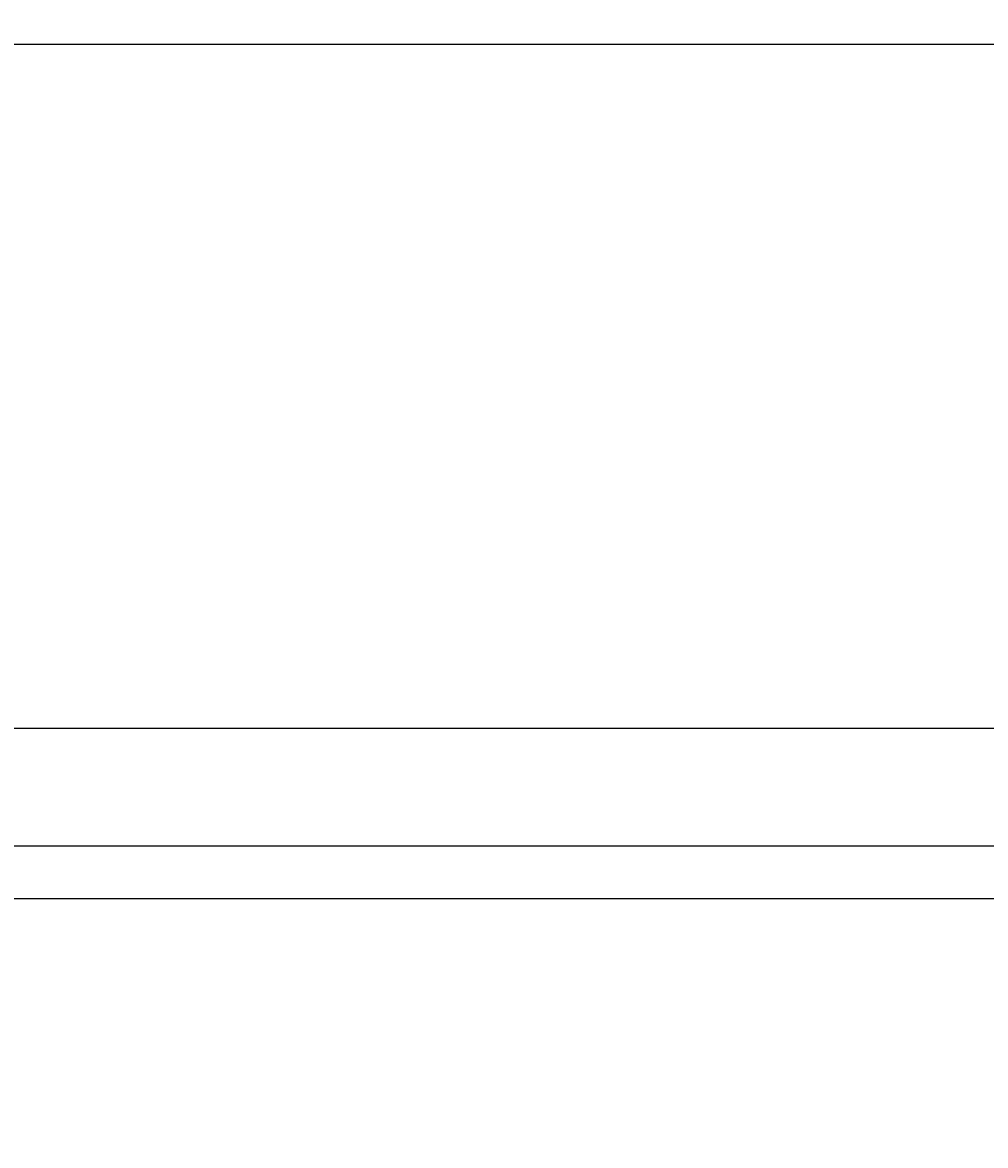
# Model space of a CAD drawing. Units: inches. Extents: x 35362 to 73946, y 43607 to 67532.
# Tile 90 of 134: x 49302 to 49711, y 48793 to 49269. Entities that reach past the tile are written whole.
import ezdxf

# ---------------------------------------------------------------- set-up
doc = ezdxf.new("R2010")
doc.units = ezdxf.units.IN
doc.header["$MEASUREMENT"] = 0
doc.layers.add('A-ANNO-DIMS', color=2, linetype='Continuous', lineweight=18)
doc.styles.get("Standard").update_dxf_attribs({"font": 'arial.ttf'})
doc.dimstyles.get("Standard").update_dxf_attribs({"dimtxt": 0.18, "dimasz": 0.18, "dimexe": 0.18, "dimexo": 0.0625, "dimgap": 0.09, "dimtad": 0, "dimtih": 1, "dimtoh": 1, "dimdec": 4, "dimzin": 0, "dimdsep": 46, "dimtxsty": 'Standard', "dimcen": 0.09, "dimadec": 0, "dimazin": 0, "dimtfac": 1, "dimtdec": 4, "dimtofl": 0, "dimtmove": 0, "dimatfit": 3, "dimfxl": 1, "dimtolj": 1, "dimtzin": 0, "dimarcsym": 0})

# ---------------------------------------------------------------- blocks, each defined once
blk = doc.blocks.new('*D11')
at = {"layer": 'A-ANNO-DIMS', "color": 0, "lineweight": -2, "transparency": 16777216}
for p, q in [((47978.66, 56028.77), (47978.66, 43606.68)), ((53109.76, 56028.77), (53109.76, 43606.68)), ((47978.84, 43606.86), (50543.87, 43606.86)), ((53109.58, 43606.86), (50544.55, 43606.86))]:
    blk.add_line(p, q, dxfattribs=at)
at = {"layer": 'A-ANNO-DIMS', "color": 0, "transparency": 16777216}
for points in [[(47978.84, 43606.89), (47978.84, 43606.83), (47978.66, 43606.86)], [(53109.58, 43606.89), (53109.58, 43606.83), (53109.76, 43606.86)]]:
    blk.add_solid(points, dxfattribs=at)
at = {"layer": 'Defpoints', "color": 0, "transparency": 16777216}
for p in [(47978.66, 56028.84), (53109.76, 56028.84), (53109.76, 43606.86)]:
    blk.add_point(p, dxfattribs=at)
at = {"layer": 'A-ANNO-DIMS', "color": 0, "transparency": 16777216, "insert": (50544.21, 43606.86), "char_height": 0.18, "attachment_point": 5}
blk.add_mtext('\\A1;5131', dxfattribs=at)
blk = doc.blocks.new('*D13')
at = {"layer": 'A-ANNO-DIMS', "color": 0, "lineweight": -2, "transparency": 16777216}
for p, q in [((48373.49, 51694.02), (48373.49, 43606.68)), ((51029.04, 51694.02), (51029.04, 43606.68)), ((48373.67, 43606.86), (49700.8, 43606.86)), ((51028.86, 43606.86), (49701.73, 43606.86))]:
    blk.add_line(p, q, dxfattribs=at)
at = {"layer": 'A-ANNO-DIMS', "color": 0, "transparency": 16777216}
for points in [[(48373.67, 43606.89), (48373.67, 43606.83), (48373.49, 43606.86)], [(51028.86, 43606.89), (51028.86, 43606.83), (51029.04, 43606.86)]]:
    blk.add_solid(points, dxfattribs=at)
at = {"layer": 'Defpoints', "color": 0, "transparency": 16777216}
for p in [(48373.49, 51694.09), (51029.04, 51694.09), (51029.04, 43606.86)]:
    blk.add_point(p, dxfattribs=at)
at = {"layer": 'A-ANNO-DIMS', "color": 0, "transparency": 16777216, "insert": (49701.27, 43606.86), "char_height": 0.18, "attachment_point": 5}
blk.add_mtext('\\A1;2655.6', dxfattribs=at)
blk = doc.blocks.new('*D67')
at = {"layer": 'A-ANNO-DIMS', "color": 0, "lineweight": -2, "transparency": 16777216}
for p, q in [((56873.54, 53351.53), (35361.77, 53351.53)), ((35361.95, 53351.35), (35361.95, 49400.89)), ((35361.95, 45450.07), (35361.95, 49400.53)), ((53793.58, 45449.89), (35361.77, 45449.89))]:
    blk.add_line(p, q, dxfattribs=at)
at = {"layer": 'A-ANNO-DIMS', "color": 0, "transparency": 16777216}
for points in [[(35361.92, 53351.35), (35361.98, 53351.35), (35361.95, 53351.53)], [(35361.92, 45450.07), (35361.98, 45450.07), (35361.95, 45449.89)]]:
    blk.add_solid(points, dxfattribs=at)
at = {"layer": 'Defpoints', "color": 0, "transparency": 16777216}
for p in [(35361.95, 53351.53), (56873.6, 53351.53), (53793.64, 45449.89)]:
    blk.add_point(p, dxfattribs=at)
at = {"layer": 'A-ANNO-DIMS', "color": 0, "transparency": 16777216, "insert": (35361.95, 49400.71), "char_height": 0.18, "attachment_point": 5}
blk.add_mtext('\\A1;7901.6', dxfattribs=at)
blk = doc.blocks.new('*D84')
at = {"layer": 'A-ANNO-DIMS', "color": 0, "lineweight": -2, "transparency": 16777216}
for p, q in [((55540.23, 49259.94), (35361.77, 49259.94)), ((35361.95, 49259.76), (35361.95, 49115.14)), ((35361.95, 48970.16), (35361.95, 49114.78)), ((55540.23, 48969.98), (35361.77, 48969.98))]:
    blk.add_line(p, q, dxfattribs=at)
at = {"layer": 'A-ANNO-DIMS', "color": 0, "transparency": 16777216}
for points in [[(35361.92, 49259.76), (35361.98, 49259.76), (35361.95, 49259.94)], [(35361.92, 48970.16), (35361.98, 48970.16), (35361.95, 48969.98)]]:
    blk.add_solid(points, dxfattribs=at)
at = {"layer": 'Defpoints', "color": 0, "transparency": 16777216}
for p in [(35361.95, 49259.94), (55540.3, 49259.94), (55540.3, 48969.98)]:
    blk.add_point(p, dxfattribs=at)
at = {"layer": 'A-ANNO-DIMS', "color": 0, "transparency": 16777216, "insert": (35361.95, 49114.96), "char_height": 0.18, "attachment_point": 5}
blk.add_mtext('\\A1;289.96', dxfattribs=at)
blk = doc.blocks.new('*D86')
at = {"layer": 'A-ANNO-DIMS', "color": 0, "lineweight": -2, "transparency": 16777216}
for p, q in [((51285.53, 49320.08), (35361.77, 49320.08)), ((35361.95, 49319.9), (35361.95, 49120.26)), ((35361.95, 48920.26), (35361.95, 49119.9)), ((51285.53, 48920.08), (35361.77, 48920.08))]:
    blk.add_line(p, q, dxfattribs=at)
at = {"layer": 'A-ANNO-DIMS', "color": 0, "transparency": 16777216}
for points in [[(35361.92, 49319.9), (35361.98, 49319.9), (35361.95, 49320.08)], [(35361.92, 48920.26), (35361.98, 48920.26), (35361.95, 48920.08)]]:
    blk.add_solid(points, dxfattribs=at)
at = {"layer": 'Defpoints', "color": 0, "transparency": 16777216}
for p in [(35361.95, 49320.08), (51285.59, 49320.08), (51285.59, 48920.08)]:
    blk.add_point(p, dxfattribs=at)
at = {"layer": 'A-ANNO-DIMS', "color": 0, "transparency": 16777216, "insert": (35361.95, 49120.08), "char_height": 0.18, "attachment_point": 5}
blk.add_mtext('\\A1;400.0', dxfattribs=at)
blk = doc.blocks.new('*D89')
at = {"layer": 'A-ANNO-DIMS', "color": 0, "lineweight": -2, "transparency": 16777216}
for p, q in [((53707.72, 48897.74), (35361.77, 48897.74)), ((35361.95, 48897.56), (35361.95, 48303.16)), ((35361.95, 47708.4), (35361.95, 48302.8)), ((53707.72, 47708.22), (35361.77, 47708.22))]:
    blk.add_line(p, q, dxfattribs=at)
at = {"layer": 'A-ANNO-DIMS', "color": 0, "transparency": 16777216}
for points in [[(35361.92, 48897.56), (35361.98, 48897.56), (35361.95, 48897.74)], [(35361.92, 47708.4), (35361.98, 47708.4), (35361.95, 47708.22)]]:
    blk.add_solid(points, dxfattribs=at)
at = {"layer": 'Defpoints', "color": 0, "transparency": 16777216}
for p in [(53707.78, 48897.74), (35361.95, 47708.22), (53707.78, 47708.22)]:
    blk.add_point(p, dxfattribs=at)
at = {"layer": 'A-ANNO-DIMS', "color": 0, "transparency": 16777216, "insert": (35361.95, 48302.98), "char_height": 0.18, "attachment_point": 5}
blk.add_mtext('\\A1;1189.5', dxfattribs=at)

msp = doc.modelspace()

# ---------------------------------------------------------------- dimensions: what is measured, and where the dimension line sits
at = {"layer": 'A-ANNO-DIMS'}
for base, p1, p2, override, picture, middle in [((53109.76, 43606.859), (47978.665, 56028.836), (53109.76, 56028.836), {"dimdec": 0, "dimlfac": 1, "dimrnd": 0, "dimzin": 0, "dimdsep": 46, "dimlunit": 2}, '*D11', (50544.212, 43606.859)), ((51029.043, 43606.859), (48373.492, 51694.087), (51029.043, 51694.087), {"dimdec": 1, "dimlfac": 1, "dimrnd": 0, "dimzin": 0, "dimdsep": 46, "dimlunit": 2}, '*D13', (49701.267, 43606.859))]:
    dim = msp.add_linear_dim(base=base, p1=p1, p2=p2, dimstyle='Standard', override=override, dxfattribs=at)
    dim.commit()
    dim.dimension.update_dxf_attribs({"geometry": picture, "text_midpoint": middle})
for base, p1, p2, override, picture, middle in [((35361.949, 53351.529), (53793.638, 45449.894), (56873.602, 53351.529), {"dimdec": 1, "dimlfac": 1, "dimrnd": 0, "dimzin": 0, "dimdsep": 46, "dimlunit": 2}, '*D67', (35361.949, 49400.712)), ((35361.949, 49320.079), (51285.595, 48920.079), (51285.595, 49320.079), {"dimdec": 1, "dimlfac": 1, "dimrnd": 0, "dimzin": 0, "dimdsep": 46, "dimlunit": 2}, '*D86', (35361.949, 49120.079)), ((35361.9491, 49259.9353), (55540.2972, 48969.9796), (55540.2972, 49259.9353), {"dimdec": 2, "dimlfac": 1, "dimrnd": 0, "dimzin": 0, "dimdsep": 46, "dimlunit": 2}, '*D84', (35361.9491, 49114.9575)), ((35361.949, 47708.216), (53707.781, 48897.738), (53707.781, 47708.216), {"dimdec": 1, "dimlfac": 1, "dimrnd": 0, "dimzin": 0, "dimdsep": 46, "dimlunit": 2}, '*D89', (35361.949, 48302.977))]:
    dim = msp.add_linear_dim(base=base, p1=p1, p2=p2, angle=90, dimstyle='Standard', override=override, dxfattribs=at)
    dim.commit()
    dim.dimension.update_dxf_attribs({"geometry": picture, "text_midpoint": middle})

doc.saveas('drawing.dxf')
